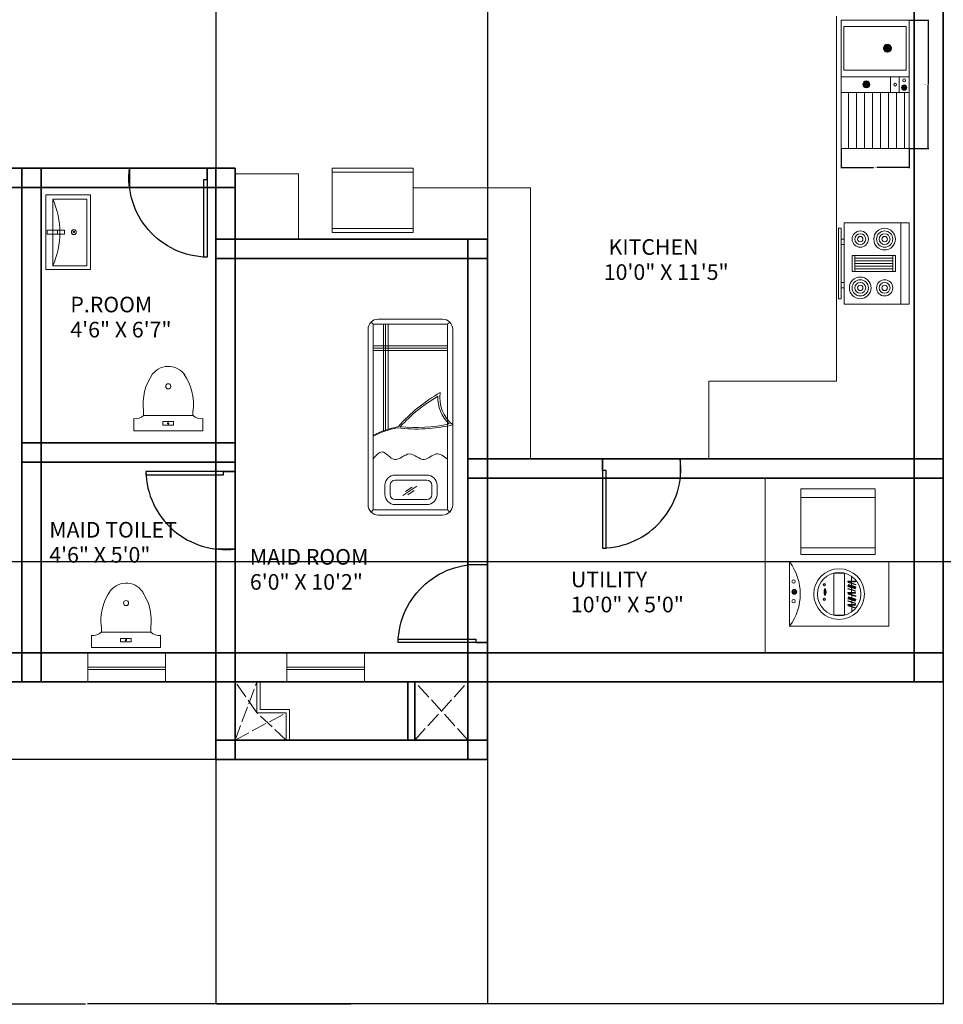
# Model space of a CAD drawing. Units: inches. Extents: x -61 to 1599, y -1316 to 257.
# Tile 20 of 204: x 259 to 545, y -1316 to -1011. Entities that reach past the tile are written whole.
import ezdxf

# ---------------------------------------------------------------- set-up
doc = ezdxf.new("R2010")
doc.units = ezdxf.units.IN
doc.header["$MEASUREMENT"] = 0
doc.linetypes.add('ACAD_ISO02W100', pattern=[15, 12, -3])
for name, color, linetype, lineweight in [('A-ANNO-DIMS', 2, 'Continuous', 18), ('A-AREA-IDEN', 1, 'Continuous', 18), ('A-EQPM', 9, 'Continuous', 18), ('A-FLOR-CASE', 8, 'Continuous', 18), ('A-FLOR-FIXT', 8, 'Continuous', 18), ('A-FLOR-OPEN-HIDN', 8, 'ACAD_ISO02W100', 13), ('A-WALL-JAMB', 4, 'ACAD_ISO02W100', 25), ('DOORS', 2, 'Continuous', 25), ('FURNITURE', 83, 'Continuous', 18), ('WALLS', 4, 'Continuous', 35), ('WINDOWS', 220, 'Continuous', 18)]:
    doc.layers.add(name, color=color, linetype=linetype, lineweight=lineweight)
doc.layers.add('FUR', color=83, linetype='Continuous')
doc.styles.get("Standard").update_dxf_attribs({"font": 'arial.ttf'})
doc.dimstyles.get("Standard").update_dxf_attribs({"dimtxt": 0.18, "dimasz": 0.18, "dimexe": 0.18, "dimexo": 0.0625, "dimgap": 0.09, "dimtad": 0, "dimtih": 1, "dimtoh": 1, "dimdec": 0, "dimzin": 0, "dimdsep": 46, "dimlunit": 3, "dimtxsty": 'Standard', "dimcen": 0.09, "dimadec": 0, "dimazin": 0, "dimtfac": 1, "dimtdec": 0, "dimtofl": 0, "dimtmove": 0, "dimatfit": 3, "dimfxl": 1, "dimtolj": 1, "dimtzin": 0, "dimarcsym": 0})

# ---------------------------------------------------------------- blocks, each defined once
blk = doc.blocks.new('Range-Oven - 30 in top')
for p, q in [((0, -3), (30, -3)), ((12, -6), (18, -6)), ((13, -20), (13, -6)), ((14, -6), (14, -20)), ((15, -20), (15, -6)), ((16, -6), (16, -20)), ((17, -20), (17, -6)), ((18, -20), (12, -20)), ((6, -24), (6, -25)), ((8, -25), (8, -24)), ((22, -25), (22, -24)), ((24, -24), (24, -25))]:
    blk.add_line(p, q)
for points in [[(0, -24), (0, 0), (30, 0), (30, -24)], [(12, -21), (12, -5), (18, -5), (18, -21)], [(2, -26), (2, -25), (28, -25), (28, -26)]]:
    blk.add_lwpolyline(points, close=True)
for centre, radius in [((6, -9), 4), ((6, -9), 3), ((6, -9), 2), ((24, -9), 3), ((24, -9), 2), ((6, -9), 1), ((24, -9), 1), ((24, -18), 4), ((6, -18), 3), ((6, -18), 2), ((6, -18), 1), ((24, -18), 3), ((24, -18), 2), ((24, -18), 1)]:
    blk.add_circle(centre, radius)
blk = doc.blocks.new('DOOR-SWING-24')
blk.add_line((0, 0), (0, 3.6))
blk.add_lwpolyline([(0, 0), (0, -24), (1.05, -24), (1.05, 0)], close=True)
blk.add_arc((-0.44, 0.62), 24.62, 271.0259, 6.9559)
blk = doc.blocks.new('WIN-24IN')
for p, q in [((0, 4.5), (0, 9)), ((0, 9), (0, 0)), ((24, 9), (24, 0)), ((0, 5.19), (24, 5.19)), ((0, 4.5), (24, 4.5))]:
    blk.add_line(p, q)
blk = doc.blocks.new('WC-FLOOR-MOUNT')
for p, q in [((3.02, 4.69), (3.02, 6.17)), ((18.31, 4.69), (18.31, 6.17)), ((0, 0), (0, 3.75)), ((3.02, 4.69), (18.31, 4.69)), ((21.33, 0), (21.33, 3.75)), ((0, 0), (21.33, 0))]:
    blk.add_line(p, q)
blk.add_lwpolyline([(12.24, 1.73), (8.96, 1.73), (8.96, 2.81), (12.24, 2.81)], close=True)
for centre, radius in [((10.67, 13.73), 0.792), ((10.6, 2.27), 0.208)]:
    blk.add_circle(centre, radius)
for centre, radius, start, end in [((10.67, 13.73), 6.18, 27.6844, 141.4697), ((19.05, 8.26), 16.17, 144.824, 187.4232), ((2.28, 8.26), 16.17, 352.5768, 35.176), ((0.56, 7.25), 3.55, 260.8586, 313.6993), ((20.77, 7.25), 3.55, 226.3007, 279.1414)]:
    blk.add_arc(centre, radius, start, end)
blk = doc.blocks.new('LAVATORY-WALL-2')
blk.add_line((3.67, 10.96), (3.67, 12.19))
for points in [[(0, 23.07), (13.87, 23.07), (13.87, 0), (0, 0)], [(12.66, 21.73), (12.66, 1.19), (2.2, 1.19), (2.2, 21.73)], [(5.78, 12.19), (5.78, 10.96), (0.4, 10.96), (0.4, 12.19)]]:
    blk.add_lwpolyline(points, close=True)
for radius in [0.74, 0.233]:
    blk.add_circle((8.7, 11.57), radius)
blk.add_arc((-20.86, 11.46), 25.25, 335.9939, 24.0061)
blk = doc.blocks.new('*U268')
at = {"layer": 'FUR'}
blk.add_line((0.41, 1.36), (0.41, 0.68), dxfattribs=at)
blk.add_open_spline([(0.41, 1.36), (0.24, 1.25), (-0.09, 1.02), (0.41, 0.7), (0.83, 0.34), (0.55, 0.11), (0.41, 0)], degree=3, knots=[0, 0, 0, 0, 0.474547, 0.949094, 1.393355, 1.837616, 1.837616, 1.837616, 1.837616], dxfattribs=at)
blk = doc.blocks.new('*U269')
at = {"layer": 'FUR', "transparency": 16777216}
for p, rotation in [((531.82, -257.55), 308.5714285714286), ((532.89, -258.18), 51.42857142857144), ((532.03, -256.89), 257.1428571428571), ((533.36, -257.68), 102.8571428571428), ((532.68, -256.65), 205.7142857142857), ((533.27, -257), 154.2857142857143)]:
    blk.add_blockref('*U268', p, dxfattribs=dict(at, rotation=rotation))
blk.add_blockref('*U268', (532.2, -258.12), dxfattribs=at)
blk = doc.blocks.new('*U270')
at = {"layer": 'FUR'}
blk.add_line((0.74, 2.46), (0.74, 1.23), dxfattribs=at)
blk.add_open_spline([(0.74, 2.46), (0.44, 2.26), (-0.16, 1.84), (0.74, 1.26), (1.5, 0.61), (0.99, 0.2), (0.74, 0)], degree=3, knots=[0, 0, 0, 0, 0.85637, 1.712739, 2.514455, 3.316171, 3.316171, 3.316171, 3.316171], dxfattribs=at)
blk = doc.blocks.new('*U271')
at = {"layer": 'FUR', "transparency": 16777216}
for p, rotation in [((959.72, -464.77), 308.5714285714286), ((961.65, -465.92), 51.42857142857144), ((960.11, -463.59), 257.1428571428571), ((962.51, -465.02), 102.8571428571428), ((961.27, -463.15), 205.7142857142858), ((962.34, -463.79), 154.2857142857143)]:
    blk.add_blockref('*U270', p, dxfattribs=dict(at, rotation=rotation))
blk.add_blockref('*U270', (960.41, -465.81), dxfattribs=at)
blk = doc.blocks.new('*U266')
at = {"layer": 'FUR'}
blk.add_line((0.41, 1.36), (0.41, 0.68), dxfattribs=at)
blk.add_open_spline([(0.41, 1.36), (0.24, 1.25), (-0.09, 1.02), (0.41, 0.7), (0.83, 0.34), (0.55, 0.11), (0.41, 0)], degree=3, knots=[0, 0, 0, 0, 0.474547, 0.949094, 1.393355, 1.837616, 1.837616, 1.837616, 1.837616], dxfattribs=at)
blk = doc.blocks.new('*U267')
at = {"layer": 'FUR', "transparency": 16777216}
for p, rotation in [((531.82, -257.55), 308.5714285714286), ((532.89, -258.18), 51.42857142857144), ((532.03, -256.89), 257.1428571428571), ((533.36, -257.68), 102.8571428571428), ((532.68, -256.65), 205.7142857142857), ((533.27, -257), 154.2857142857143)]:
    blk.add_blockref('*U266', p, dxfattribs=dict(at, rotation=rotation))
blk.add_blockref('*U266', (532.2, -258.12), dxfattribs=at)
blk = doc.blocks.new('SINK-WITH-DRAINBOARD')
for p, q in [((14.29, 30.97), (14.29, 29.74)), ((0, 22.17), (20.98, 22.17)), ((15.24, 17.27), (15.24, 22.17)), ((17.97, 22.17), (17.97, 17.27)), ((7.79, 19.82), (7.79, 19.14)), ((19.48, 18.8), (19.48, 18.12)), ((0, 17.27), (20.98, 17.27)), ((2.27, 0), (2.27, 17.27)), ((4.74, 0), (4.74, 17.27)), ((7.21, 0), (7.21, 17.27)), ((9.69, 0), (9.69, 17.27)), ((12.16, 0), (12.16, 17.27)), ((14.63, 0), (14.63, 17.27)), ((17.1, 0), (17.1, 17.27)), ((19.58, 0), (19.58, 17.27))]:
    blk.add_line(p, q)
for points in [[(20.98, 0), (0, 0), (0, 39.63), (20.98, 39.63)], [(20.07, 24.22), (0.86, 24.22), (0.86, 37.7), (20.07, 37.7)]]:
    blk.add_lwpolyline(points, close=True)
for centre, radius in [((14.29, 30.97), 1.23), ((19.48, 21.05), 0.455), ((7.78, 19.81), 1.08), ((7.78, 19.81), 0.877), ((7.79, 19.82), 0.682), ((16.69, 19.72), 0.419), ((19.48, 18.8), 0.816), ((19.48, 18.8), 0.816), ((19.48, 18.8), 0.682)]:
    blk.add_circle(centre, radius)
for name, p in [('*U271', (-946.85, 495.54)), ('*U269', (-524.82, 277.26)), ('*U267', (-513.12, 276.24))]:
    blk.add_blockref(name, p)
blk = doc.blocks.new('UTILITY-CABINET')
for p, q in [((0, 17.69), (23.01, 17.69)), ((0, 2.1), (23.01, 2.1))]:
    blk.add_line(p, q)
blk.add_lwpolyline([(23.01, 0), (0, 0), (0, 20.31), (23.01, 20.31)], close=True)
blk = doc.blocks.new('KITCHEN-BASE-UNIT')
for p, q in [((25.07, 18.6), (0, 18.6)), ((25.07, 1.23), (0, 1.23))]:
    blk.add_line(p, q)
blk.add_lwpolyline([(25.07, 0), (0, 0), (0, 19.92), (25.07, 19.92)], close=True)
blk = doc.blocks.new('*D656')
at = {"layer": 'A-ANNO-DIMS', "color": 0, "lineweight": -2, "transparency": 16777216}
for p, q in [((534.16, -1011.24), (540.23, -1011.24)), ((540.05, -1011.42), (540.05, -1030.87)), ((540.05, -1050.69), (540.05, -1031.24)), ((534.16, -1050.87), (540.23, -1050.87))]:
    blk.add_line(p, q, dxfattribs=at)
at = {"layer": 'A-ANNO-DIMS', "color": 0, "transparency": 16777216}
for points in [[(540.02, -1011.42), (540.08, -1011.42), (540.05, -1011.24)], [(540.02, -1050.69), (540.08, -1050.69), (540.05, -1050.87)]]:
    blk.add_solid(points, dxfattribs=at)
at = {"layer": 'DEFPOINTS', "color": 0, "transparency": 16777216}
for p in [(534.1, -1011.24), (540.05, -1011.24), (534.1, -1050.87)]:
    blk.add_point(p, dxfattribs=at)
at = {"layer": 'A-ANNO-DIMS', "color": 0, "transparency": 16777216, "insert": (540.05, -1031.05), "char_height": 0.18, "attachment_point": 5}
blk.add_mtext('\\A1;KITCHEN SINK 40 TYP.', dxfattribs=at)
blk = doc.blocks.new('*D657')
at = {"layer": 'A-ANNO-DIMS', "color": 0, "lineweight": -2, "transparency": 16777216}
for p, q in [((513.13, -1050.93), (513.13, -1056.99)), ((534.1, -1050.93), (534.1, -1056.99)), ((513.31, -1056.81), (523.08, -1056.81)), ((533.92, -1056.81), (524.14, -1056.81))]:
    blk.add_line(p, q, dxfattribs=at)
at = {"layer": 'A-ANNO-DIMS', "color": 0, "transparency": 16777216}
for points in [[(513.31, -1056.78), (513.31, -1056.84), (513.13, -1056.81)], [(533.92, -1056.78), (533.92, -1056.84), (534.1, -1056.81)]]:
    blk.add_solid(points, dxfattribs=at)
at = {"layer": 'DEFPOINTS', "color": 0, "transparency": 16777216}
for p in [(513.13, -1050.87), (534.1, -1050.87), (534.1, -1056.81)]:
    blk.add_point(p, dxfattribs=at)
at = {"layer": 'A-ANNO-DIMS', "color": 0, "transparency": 16777216, "insert": (523.61, -1056.81), "char_height": 0.18, "attachment_point": 5}
blk.add_mtext('\\A1;21 TYP.', dxfattribs=at)
blk = doc.blocks.new('*D687')
at = {"layer": 'A-ANNO-DIMS', "color": 0, "lineweight": -2, "transparency": 16777216}
for p, q in [((289.42, 181.68), (-61.08, 181.68)), ((-60.9, 181.5), (-60.9, -528.95)), ((-60.9, -1239.76), (-60.9, -529.32)), ((319.64, -1239.94), (-61.08, -1239.94))]:
    blk.add_line(p, q, dxfattribs=at)
at = {"layer": 'A-ANNO-DIMS', "color": 0, "transparency": 16777216}
for points in [[(-60.93, 181.5), (-60.87, 181.5), (-60.9, 181.68)], [(-60.93, -1239.76), (-60.87, -1239.76), (-60.9, -1239.94)]]:
    blk.add_solid(points, dxfattribs=at)
at = {"layer": 'DEFPOINTS', "color": 0, "transparency": 16777216}
for p in [(289.48, 181.68), (-60.9, -1239.94), (319.7, -1239.94)]:
    blk.add_point(p, dxfattribs=at)
at = {"layer": 'A-ANNO-DIMS', "color": 0, "transparency": 16777216, "insert": (-60.9, -529.13), "char_height": 0.18, "attachment_point": 5}
blk.add_mtext('\\A1;1421.6', dxfattribs=at)
blk = doc.blocks.new('*D688')
at = {"layer": 'A-ANNO-DIMS', "color": 0, "lineweight": -2, "transparency": 16777216}
for p, q in [((14.7, -1216.01), (14.7, -1315.72)), ((544.7, -1216.01), (544.7, -1315.72)), ((14.88, -1315.54), (279.41, -1315.54)), ((544.52, -1315.54), (279.99, -1315.54))]:
    blk.add_line(p, q, dxfattribs=at)
at = {"layer": 'A-ANNO-DIMS', "color": 0, "transparency": 16777216}
for points in [[(14.88, -1315.51), (14.88, -1315.57), (14.7, -1315.54)], [(544.52, -1315.51), (544.52, -1315.57), (544.7, -1315.54)]]:
    blk.add_solid(points, dxfattribs=at)
at = {"layer": 'DEFPOINTS', "color": 0, "transparency": 16777216}
for p in [(14.7, -1215.94), (544.7, -1215.94), (544.7, -1315.54)]:
    blk.add_point(p, dxfattribs=at)
at = {"layer": 'A-ANNO-DIMS', "color": 0, "transparency": 16777216, "insert": (279.7, -1315.54), "char_height": 0.18, "attachment_point": 5}
blk.add_mtext('\\A1;530', dxfattribs=at)
blk = doc.blocks.new('*D696')
at = {"layer": 'A-ANNO-DIMS', "color": 0, "lineweight": -2, "transparency": 16777216}
for p, q in [((690.64, -873.17), (-61.08, -873.17)), ((-60.9, -873.35), (-60.9, -1025.8)), ((-60.9, -1178.61), (-60.9, -1026.16)), ((690.64, -1178.79), (-61.08, -1178.79))]:
    blk.add_line(p, q, dxfattribs=at)
at = {"layer": 'A-ANNO-DIMS', "color": 0, "transparency": 16777216}
for points in [[(-60.93, -873.35), (-60.87, -873.35), (-60.9, -873.17)], [(-60.93, -1178.61), (-60.87, -1178.61), (-60.9, -1178.79)]]:
    blk.add_solid(points, dxfattribs=at)
at = {"layer": 'DEFPOINTS', "color": 0, "transparency": 16777216}
for p in [(-60.9, -873.17), (690.7, -873.17), (690.7, -1178.79)]:
    blk.add_point(p, dxfattribs=at)
at = {"layer": 'A-ANNO-DIMS', "color": 0, "transparency": 16777216, "insert": (-60.9, -1025.98), "char_height": 0.18, "attachment_point": 5}
blk.add_mtext('\\A1;305.6', dxfattribs=at)
blk = doc.blocks.new('*D710')
at = {"layer": 'A-ANNO-DIMS', "color": 0, "lineweight": -2, "transparency": 16777216}
for p, q in [((319.7, -465.39), (319.7, -1315.72)), ((403.7, -465.39), (403.7, -1315.72)), ((319.88, -1315.54), (361.48, -1315.54)), ((403.52, -1315.54), (361.92, -1315.54))]:
    blk.add_line(p, q, dxfattribs=at)
at = {"layer": 'A-ANNO-DIMS', "color": 0, "transparency": 16777216}
for points in [[(319.88, -1315.51), (319.88, -1315.57), (319.7, -1315.54)], [(403.52, -1315.51), (403.52, -1315.57), (403.7, -1315.54)]]:
    blk.add_solid(points, dxfattribs=at)
at = {"layer": 'DEFPOINTS', "color": 0, "transparency": 16777216}
for p in [(319.7, -465.32), (403.7, -465.32), (403.7, -1315.54)]:
    blk.add_point(p, dxfattribs=at)
at = {"layer": 'A-ANNO-DIMS', "color": 0, "transparency": 16777216, "insert": (361.7, -1315.54), "char_height": 0.18, "attachment_point": 5}
blk.add_mtext('\\A1;84', dxfattribs=at)

msp = doc.modelspace()

# ---------------------------------------------------------------- linework, layer by layer
at = {"layer": 'A-EQPM'}
for p, q in [((516.3756, -1194.2477), (516.3533, -1183.3071)), ((498.1109, -1188.0836), (497.8816, -1188.0836)), ((498.0958, -1187.5619), (498.2589, -1187.7231)), ((498.6238, -1187.3414), (498.6238, -1187.5707)), ((499.1556, -1187.5657), (498.9913, -1187.7257)), ((499.3661, -1188.0836), (499.1368, -1188.0836)), ((508.1302, -1189.2539), (508.1302, -1187.0404)), ((498.2564, -1188.4415), (498.0921, -1188.6014)), ((498.6238, -1188.5965), (498.6238, -1188.8258)), ((498.9887, -1188.4441), (499.1518, -1188.6052))]:
    msp.add_line(p, q, dxfattribs=at)
for points in [[(527.8101, -1198.7207), (497.1329, -1198.7207), (497.1329, -1178.8499), (527.8101, -1178.8499)], [(514.1124, -1195.2958), (510.8306, -1195.2958), (510.8306, -1182.2748), (514.1124, -1182.2748)], [(517.5666, -1184.9438), (515.1463, -1184.9438), (515.1463, -1184.7705), (517.5666, -1184.7705)], [(515.3452, -1185.0819), (517.6578, -1185.7962), (517.6067, -1185.9617), (515.2941, -1185.2475)], [(515.2257, -1186.2698), (517.5383, -1186.9841), (517.4872, -1187.1496), (515.1746, -1186.4354)], [(515.231, -1187.0142), (517.5436, -1187.7285), (517.4925, -1187.894), (515.1799, -1187.1797)], [(515.3505, -1185.8263), (517.6631, -1186.5406), (517.612, -1186.7061), (515.2994, -1185.9918)], [(517.574, -1188.493), (515.1537, -1188.493), (515.1537, -1188.3197), (517.574, -1188.3197)], [(515.2373, -1190.0933), (517.5498, -1190.8076), (517.4987, -1190.9731), (515.1861, -1190.2588)], [(515.2426, -1190.8376), (517.5551, -1191.5519), (517.504, -1191.7174), (515.1914, -1191.0032)], [(515.3526, -1188.6311), (517.6652, -1189.3454), (517.6141, -1189.5109), (515.3015, -1188.7966)], [(515.3621, -1189.6497), (517.6747, -1190.364), (517.6235, -1190.5295), (515.311, -1189.8153)], [(517.5813, -1192.1645), (515.161, -1192.1645), (515.161, -1191.9912), (517.5813, -1191.9912)], [(515.3599, -1192.3026), (517.6725, -1193.0169), (517.6214, -1193.1824), (515.3088, -1192.4682)]]:
    msp.add_lwpolyline(points, close=True, dxfattribs=at)
for centre, radius in [((512.4715, -1188.7853), 7.8534), ((512.4715, -1188.7853), 7.8534), ((512.4715, -1188.7853), 6.7141), ((498.4111, -1184.8955), 0.5265), ((498.6238, -1188.0836), 0.7422), ((498.6238, -1188.0836), 0.5129), ((498.6238, -1188.0836), 0.1784), ((498.6238, -1188.0836), 0.07), ((507.9006, -1185.8622), 0.3807), ((507.9006, -1185.8622), 0.2886), ((498.4111, -1190.9675), 0.5265), ((507.9006, -1190.4268), 0.3807), ((507.9006, -1190.4268), 0.2886)]:
    msp.add_circle(centre, radius, dxfattribs=at)
for centre, radius, start, end in [((484.0116, -1188.7853), 16.4584, 322.867122, 37.132878), ((509.931, -1188.1471), 2.1137, 148.425067, 211.574933), ((506.3294, -1188.1471), 2.1137, 328.425067, 31.574933)]:
    msp.add_arc(centre, radius, start, end, dxfattribs=at)
at = {"layer": 'A-FLOR-CASE'}
for p, q in [((511.7028, -1009.9446), (511.7028, -1033.9446)), ((511.7028, -1122.9446), (511.7028, -1033.9446)), ((380.7476, -1063.0322), (417.0519, -1063.0322)), ((417.0519, -1063.0322), (417.0519, -1146.9446)), ((511.7028, -1122.9446), (472.2349, -1122.9446)), ((472.2349, -1122.9446), (472.2349, -1146.9446)), ((489.5747, -1206.9446), (489.5747, -1152.9446))]:
    msp.add_line(p, q, dxfattribs=at)
msp.add_lwpolyline([(345.3268, -1078.9446), (325.7028, -1078.9446), (325.7028, -1058.6906), (345.3268, -1058.6906)], close=True, dxfattribs=at)
at = {"layer": 'A-FLOR-OPEN-HIDN', "ltscale": 0.4}
for p, q in [((325.7028, -1233.9446), (332.4306, -1215.9446)), ((332.4306, -1225.5432), (325.7028, -1215.9446)), ((381.272, -1233.9446), (397.7028, -1215.9446)), ((397.7028, -1233.9446), (381.272, -1215.9446)), ((325.7028, -1233.9446), (341.4965, -1225.5432)), ((341.4965, -1233.9446), (332.4306, -1225.5432))]:
    msp.add_line(p, q, dxfattribs=at)
at = {"layer": 'A-FLOR-OPEN-HIDN'}
for p, q in [((332.4306, -1215.9446), (332.4306, -1225.5432)), ((333.4306, -1215.9446), (333.4306, -1224.5432)), ((333.4306, -1224.5432), (342.4965, -1224.5432)), ((342.4965, -1224.5432), (342.4965, -1233.9446)), ((332.4306, -1225.5432), (341.4965, -1225.5432)), ((341.4965, -1225.5432), (341.4965, -1233.9446))]:
    msp.add_line(p, q, dxfattribs=at)
at = {"layer": 'A-WALL-JAMB'}
for p, q in [((293.017, -1056.9446), (293.017, -1062.9446)), ((317.017, -1056.9446), (317.017, -1062.9446)), ((439.3522, -1146.9446), (439.3522, -1152.9446)), ((463.3522, -1146.9446), (463.3477, -1152.9446)), ((325.7028, -1150.8428), (319.7028, -1150.8428)), ((325.7028, -1174.8428), (319.7028, -1174.8428)), ((403.7028, -1179.763), (397.7028, -1179.763)), ((403.7028, -1203.763), (397.7028, -1203.763))]:
    msp.add_line(p, q, dxfattribs=at)
at = {"layer": 'FURNITURE'}
for p, q in [((368.3698, -1105.2891), (367.7148, -1104.6341)), ((371.5985, -1138.276), (371.5985, -1105.2891)), ((372.1865, -1138.0647), (372.1865, -1105.2891)), ((373.0588, -1137.7759), (373.0588, -1105.2891)), ((391.4076, -1105.2891), (392.0626, -1104.6341)), ((391.4076, -1111.9301), (368.3698, -1111.9301)), ((391.4076, -1112.6394), (368.3698, -1112.6394)), ((391.4076, -1113.4088), (368.3698, -1113.4088)), ((381.8729, -1155.4098), (377.5662, -1158.2966)), ((378.3763, -1157.0091), (380.413, -1155.6521)), ((379.072, -1158.0533), (381.1087, -1156.6963)), ((368.3698, -1162.753), (367.7148, -1163.408)), ((392.0626, -1163.408), (391.4076, -1162.753))]:
    msp.add_line(p, q, dxfattribs=at)
for points in [[(369.9511, -1103.7078), (389.8263, -1103.7078, -0.41421356), (392.989, -1106.8704), (392.989, -1161.1717, -0.41421356), (389.8263, -1164.3343), (369.9511, -1164.3343, -0.41421356), (366.7885, -1161.1717), (366.7885, -1106.8704, -0.41421356)], [(375.197, -1151.9572), (384.9839, -1151.9572, -0.41421356), (388.1465, -1155.1198), (388.1465, -1157.9358, -0.41421356), (384.9839, -1161.0984), (375.197, -1161.0984, -0.41421356), (372.0344, -1157.9358), (372.0344, -1155.1198, -0.41421356)], [(375.197, -1153.5385), (384.9839, -1153.5385, -0.41421356), (386.5652, -1155.1198), (386.5652, -1157.9358, -0.41421356), (384.9839, -1159.5171), (375.197, -1159.5171, -0.41421356), (373.6157, -1157.9358), (373.6157, -1155.1198, -0.41421356)]]:
    msp.add_lwpolyline(points, format="xyb", close=True, dxfattribs=at)
msp.add_lwpolyline([(368.3698, -1105.2891), (391.4076, -1105.2891), (391.4076, -1162.753), (368.3698, -1162.753)], close=True, dxfattribs=at)
for centre, radius, start, end in [((412.8702, -1168.7842), 48.5558, 119.302799, 139.065497), ((400.0028, -1127.9647), 11.0029, 172.042189, 230.397858), ((412.7906, -1169.5476), 48.5558, 120.122754, 137.951503), ((399.4118, -1128.0987), 11.0029, 177.136894, 226.788842), ((381.953, -1089.1573), 48.5558, 262.813151, 283.137248), ((381.4332, -1088.699), 48.5558, 264.446321, 282.422187), ((382.2263, -1166.9235), 30.5553, 101.397161, 116.967867), ((381.9164, -1167.2844), 30.5553, 101.397161, 116.317614)]:
    msp.add_arc(centre, radius, start, end, dxfattribs=at)
msp.add_open_spline([(391.4076, -1147.0167), (390.2379, -1146.131), (387.818, -1144.2987), (383.9669, -1148.7668), (379.6119, -1143.5647), (375.0321, -1149.1441), (371.3585, -1143.3084), (369.2784, -1145.8454), (368.3698, -1146.9534)], degree=3, knots=[0, 0, 0, 0, 3.84254534, 7.94890144, 12.81558195, 17.74158221, 22.25649, 25.75782552, 25.75782552, 25.75782552, 25.75782552], dxfattribs=at)
at = {"layer": 'WALLS'}
for p, q in [((535.7028, -1215.9446), (535.7028, -741.169)), ((544.7028, -1215.9446), (544.7028, -741.169)), ((237.7028, -1056.9446), (325.7028, -1056.9446)), ((259.7028, -1056.9446), (259.7028, -1215.9446)), ((265.7028, -1056.9446), (265.7028, -1215.9446)), ((319.7028, -1056.9446), (319.7028, -1215.9446)), ((325.7028, -1056.9446), (325.7028, -1215.9446)), ((237.7028, -1062.9446), (325.7028, -1062.9446)), ((319.7028, -1078.9446), (403.7028, -1078.9446)), ((397.7028, -1078.9446), (397.7028, -1215.9446)), ((403.7028, -1078.9446), (403.7028, -1215.9446)), ((319.7028, -1084.9446), (403.7028, -1084.9446)), ((259.7028, -1141.9446), (325.7028, -1141.9446)), ((259.7028, -1147.9446), (325.7028, -1147.9446)), ((397.7028, -1146.9446), (544.7028, -1146.9446)), ((397.7028, -1152.9446), (544.7028, -1152.9446)), ((237.7028, -1206.9446), (327.7028, -1206.9446)), ((327.7028, -1206.9446), (403.7028, -1206.9446)), ((397.7028, -1206.9446), (544.7028, -1206.9446)), ((237.7028, -1215.9446), (327.7028, -1215.9446)), ((319.7028, -1215.9446), (319.7028, -1239.9446)), ((325.7028, -1215.9446), (325.7028, -1239.9446)), ((327.7028, -1215.9446), (403.7028, -1215.9446)), ((379.1436, -1233.9446), (379.1436, -1215.9446)), ((381.272, -1233.9446), (381.272, -1215.9446)), ((397.7028, -1215.9446), (544.7028, -1215.9446)), ((397.7028, -1215.9446), (397.7028, -1239.9446)), ((403.7028, -1215.9446), (403.7028, -1239.9446)), ((403.7028, -1233.9446), (319.7028, -1233.9446)), ((403.7028, -1239.9446), (319.7028, -1239.9446))]:
    msp.add_line(p, q, dxfattribs=at)

# ---------------------------------------------------------------- block references
at = {"layer": 'A-EQPM', "xscale": 0.8378013827109642, "yscale": 0.8378013827109642, "zscale": 0.8378013827109642, "rotation": 270}
msp.add_blockref('Range-Oven - 30 in top', (534.1022, -1073.9166), dxfattribs=at)
at = {"layer": 'A-FLOR-CASE'}
for name, p in [('KITCHEN-BASE-UNIT', (355.674, -1076.8667)), ('UTILITY-CABINET', (500.634, -1176.5377))]:
    msp.add_blockref(name, p, dxfattribs=at)
at = {"layer": 'A-FLOR-FIXT'}
for name, p in [('SINK-WITH-DRAINBOARD', (513.125, -1050.8657)), ('LAVATORY-WALL-2', (267.1172, -1088.3512)), ('WC-FLOOR-MOUNT', (294.349, -1138.2323)), ('WC-FLOOR-MOUNT', (281.2982, -1205.2969))]:
    msp.add_blockref(name, p, dxfattribs=at)
at = {"layer": 'DOORS', "extrusion": (0, 0, -1), "zscale": -1}
msp.add_blockref('DOOR-SWING-24', (-317.017, -1060.5446), dxfattribs=at)
at = {"layer": 'DOORS'}
msp.add_blockref('DOOR-SWING-24', (439.3522, -1150.5446), dxfattribs=at)
at = {"layer": 'DOORS', "rotation": 270.0000000000007}
msp.add_blockref('DOOR-SWING-24', (322.1028, -1150.8428), dxfattribs=at)
at = {"layer": 'DOORS', "extrusion": (0, 0, -1), "zscale": -1, "rotation": 89.99999999999984}
msp.add_blockref('DOOR-SWING-24', (-400.1028, -1203.763), dxfattribs=at)
at = {"layer": 'WINDOWS', "rotation": 180}
for p in [(304.1139, -1206.9445), (365.7033, -1206.9445)]:
    msp.add_blockref('WIN-24IN', p, dxfattribs=at)

# ---------------------------------------------------------------- texts
at = {"layer": 'A-AREA-IDEN'}
for s, height, p in [(' KITCHEN', 4.8321, (439.7144, -1083.8048)), ('10\'0" X 11\'5"', 4.832098, (439.7144, -1091.5671)), ('P.ROOM', 4.8321, (274.7407, -1101.5989)), ('4\'6" X 6\'7"', 4.832098, (274.7407, -1109.3612)), ('MAID TOILET', 4.832098, (268.2172, -1171.2898)), ('4\'6" X 5\'0"', 4.832098, (268.2172, -1179.0521)), ('MAID ROOM', 4.8321, (330.2598, -1179.6775)), ('UTILITY', 4.8321, (429.5332, -1186.6671)), ('6\'0" X 10\'2"', 4.832098, (330.2598, -1187.4399)), ('10\'0" X 5\'0"', 4.832098, (429.5332, -1194.4295))]:
    msp.add_text(s, height=height, dxfattribs=at).set_placement(p)

# ---------------------------------------------------------------- dimensions: what is measured, and where the dimension line sits
at = {"layer": 'A-ANNO-DIMS'}
for base, p1, p2, picture, middle in [((-60.8972, -1239.9446), (289.4807, 181.6771), (319.7028, -1239.9446), '*D687', (-60.8972, -529.1337)), ((-60.8972, -873.169), (690.7028, -1178.7933), (690.7028, -873.169), '*D696', (-60.8972, -1025.9812))]:
    dim = msp.add_linear_dim(base=base, p1=p1, p2=p2, angle=90, dimstyle='Standard', override={"dimdec": 1, "dimlfac": 1, "dimrnd": 0, "dimzin": 0, "dimdsep": 46, "dimlunit": 2}, dxfattribs=at)
    dim.commit()
    dim.dimension.update_dxf_attribs({"geometry": picture, "text_midpoint": middle})
for base, p1, p2, picture, middle in [((403.7028, -1315.5446), (319.7028, -465.3229), (403.7028, -465.3229), '*D710', (361.7028, -1315.5446)), ((544.7028, -1315.5446), (14.7028, -1215.9446), (544.7028, -1215.9446), '*D688', (279.7028, -1315.5446))]:
    dim = msp.add_linear_dim(base=base, p1=p1, p2=p2, dimstyle='Standard', override={"dimdec": 0, "dimlfac": 1, "dimrnd": 0, "dimzin": 0, "dimdsep": 46, "dimlunit": 2}, dxfattribs=at)
    dim.commit()
    dim.dimension.update_dxf_attribs({"geometry": picture, "text_midpoint": middle})
dim = msp.add_linear_dim(base=(540.0462, -1011.2397), p1=(534.1022, -1050.8661), p2=(534.1022, -1011.2397), angle=90, text='KITCHEN SINK <> TYP.', dimstyle='Standard', override={"dimdec": 0, "dimlfac": 1, "dimrnd": 0, "dimzin": 0, "dimdsep": 46, "dimlunit": 2}, dxfattribs=at)
dim.commit()
dim.dimension.update_dxf_attribs({"geometry": '*D656', "text_midpoint": (540.0462, -1031.0529)})
dim = msp.add_linear_dim(base=(534.1022, -1056.8101), p1=(513.125, -1050.8661), p2=(534.1022, -1050.8661), text='<> TYP.', dimstyle='Standard', override={"dimdec": 0, "dimlfac": 1, "dimrnd": 0, "dimzin": 0, "dimdsep": 46, "dimlunit": 2}, dxfattribs=at)
dim.commit()
dim.dimension.update_dxf_attribs({"geometry": '*D657', "text_midpoint": (523.6136, -1056.8101)})

doc.saveas('drawing.dxf')
